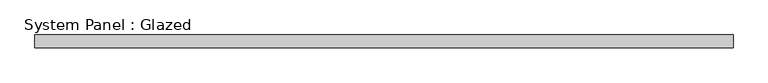
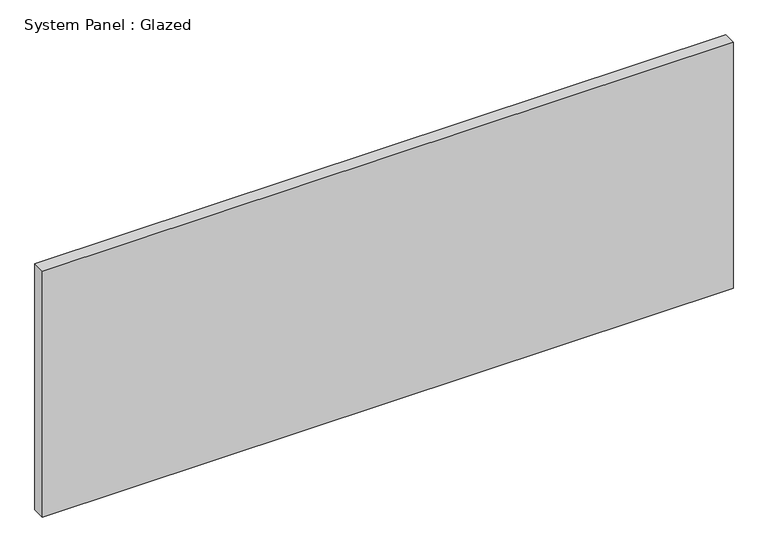
"""IFC4 building model written with IfcOpenShell, lengths in millimetres: plate geometry, System Panel : Glazed."""

from ifc_helpers import new_model, si_unit, origin, origin_with_axes, place, context, project, spatial, polyline, outline, extrude, source, transform, mapped, element, save


def system_panel_glazed_2a82d765(model_context):
    return source(origin(), model_context, "Body", "SweptSolid", [
        extrude(outline(polyline([(683.0342567, 19.05), (-683.0342567, 19.05), (-683.0342567, 44.45), (683.0342567, 44.45), (683.0342567, 19.05)])), origin_with_axes(), (0.0, 0.0, 1.0), 514.35),
    ])


if __name__ == "__main__":
    model = new_model("IFC4")
    model_context = context("Model", 3, world=origin())
    ifc_project = project(units=[si_unit("LENGTHUNIT", "METRE", prefix="MILLI")], contexts=[model_context])
    site = spatial("IfcSite", under=ifc_project)
    building = spatial("IfcBuilding", under=site)
    placement = place(None, origin())
    system_panel_glazed_shape = system_panel_glazed_2a82d765(model_context)
    element("IfcPlate", 1, ObjectType="System Panel : Glazed", at=placement, inside=building, context=model_context, shape_type="MappedRepresentation", body=[
        mapped(system_panel_glazed_shape, transform((0.0, 0.0, 0.0), x_axis=(1.0, 0.0, 0.0), y_axis=(0.0, 1.0, 0.0), z_axis=(0.0, 0.0, 1.0))),
    ])
    save(model, "model.ifc")

# Revit data of these elements
# Type "System Panel : Glazed"
#   Construction Type Id = "GSP4R"
#   Analytic Construction = "1/8 in Pilkington single glazing"
#   Visual Light Transmittance = 0.9
#   Solar Heat Gain Coefficient = 0.86
#   Heat Transfer Coefficient (U) = 1.18115 BTU/(h·ft²·°F)
# Element 1 (IfcPlate, "System Panel : Glazed")
#   Materials on its faces: "Glass"
# Materials
#   "Glass": class "Glass", colour RGB 0 128 192, transparency 0.75, Description = "Soda Lime Glass", Cost = 0
